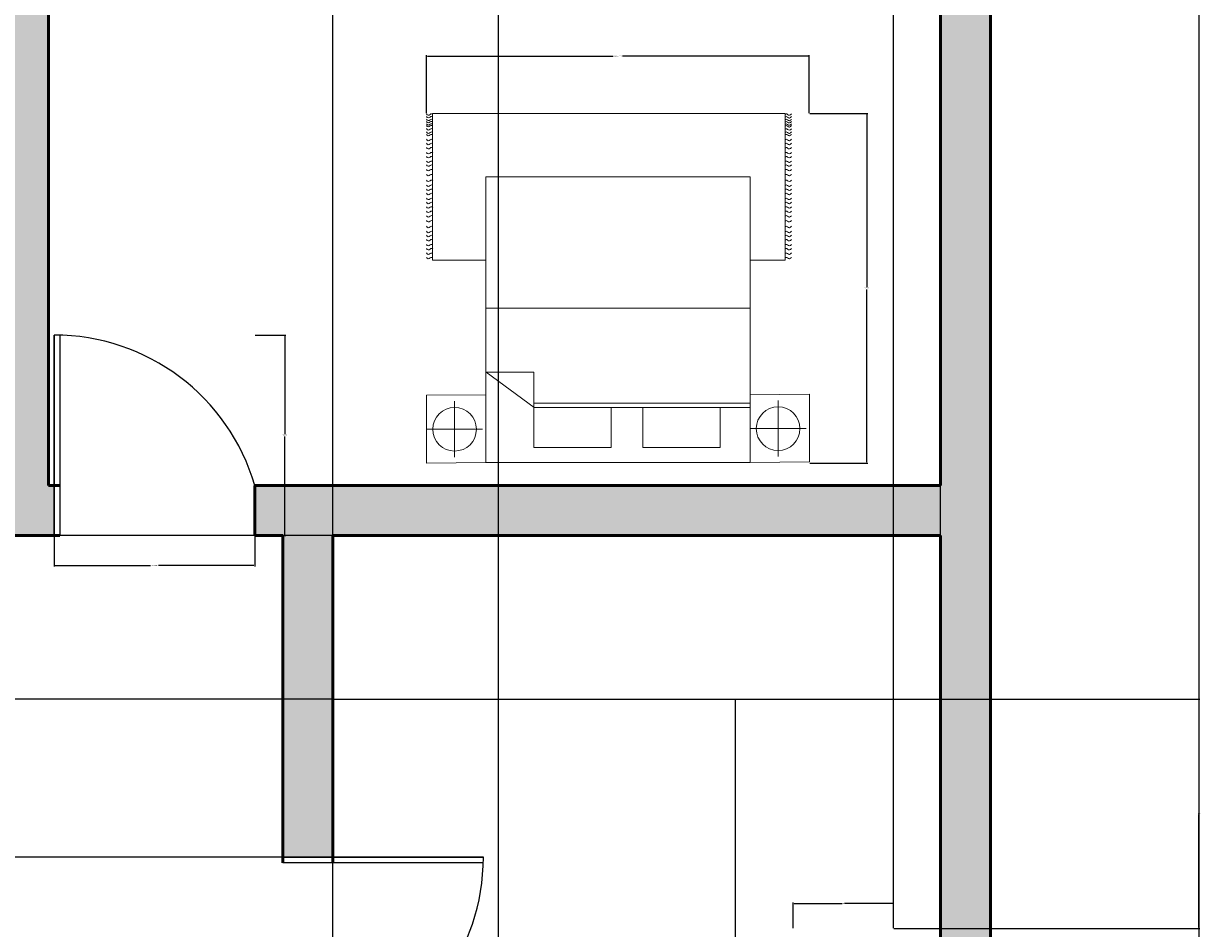
# Model space of a CAD drawing. Units: inches. Extents: x 383 to 970, y 275 to 1088.
# Tile 10 of 11: x 759 to 970, y 713 to 875. Entities that reach past the tile are written whole.
import ezdxf

# ---------------------------------------------------------------- set-up
doc = ezdxf.new("R2010")
doc.units = ezdxf.units.IN
doc.header["$MEASUREMENT"] = 0
for name, color, linetype, lineweight in [('A-ANNO-DIMS', 2, 'Continuous', 18), ('A-DOOR', 3, 'Continuous', 25), ('A-FLOR-CASE', 8, 'Continuous', 25), ('A-FURN', 8, 'Continuous', 18), ('A-WALL', 7, 'Continuous', 50)]:
    doc.layers.add(name, color=color, linetype=linetype, lineweight=lineweight)
doc.layers.add('A-WALL-PATT', color=251, linetype='Continuous', lineweight=13, true_color=0x636466)
doc.styles.get("Standard").update_dxf_attribs({"font": 'arial.ttf'})
doc.dimstyles.get("Standard").update_dxf_attribs({"dimtxt": 0.18, "dimasz": 0.18, "dimexe": 0.18, "dimexo": 0.0625, "dimgap": 0.09, "dimtad": 0, "dimtih": 1, "dimtoh": 1, "dimdec": 4, "dimzin": 0, "dimdsep": 46, "dimtxsty": 'Standard', "dimcen": 0.09, "dimadec": 0, "dimazin": 0, "dimtfac": 1, "dimtdec": 4, "dimtofl": 0, "dimtmove": 0, "dimatfit": 3, "dimfxl": 1, "dimtolj": 1, "dimtzin": 0, "dimarcsym": 0})

# ---------------------------------------------------------------- blocks, each defined once
blk = doc.blocks.new('BED-DOUBLE-WITH-NIGHTSTANDS')
for p, q in [((6.09, 68.68), (6.09, 58.62)), ((36.42, 67.59), (62.78, 67.59)), ((36.42, 58.05), (36.42, 67.59)), ((62.78, 67.59), (62.78, 4.35)), ((1.07, 63.65), (11.12, 63.65)), ((9.97, 49.39), (16.32, 58)), ((16.32, 49.44), (16.32, 58)), ((27.82, 58.05), (27.82, 10.63)), ((9.97, 49.44), (16.32, 49.44)), ((9.97, 49.39), (9.97, 10.63)), ((10.78, 49.44), (10.78, 10.63)), ((6.2, 10.63), (6.2, 0.57)), ((36.42, 4.35), (36.42, 10.65)), ((1.17, 5.6), (11.22, 5.6)), ((62.78, 4.35), (36.42, 4.35))]:
    blk.add_line(p, q)
for points in [[(12.29, 58.05), (12.19, 68.68), (0, 68.68), (0.1, 58.05)], [(0.1, 58.05), (51.42, 58.05), (51.42, 10.63), (0.1, 10.63)], [(2.8, 49.44), (9.97, 49.44), (9.97, 35.55), (2.8, 35.55)], [(2.8, 29.88), (9.97, 29.88), (9.97, 15.98), (2.8, 15.98)], [(12.39, 0), (12.29, 10.63), (0.1, 10.63), (0.21, 0)]]:
    blk.add_lwpolyline(points, close=True)
for centre in [(6.09, 63.65), (6.2, 5.6)]:
    blk.add_circle(centre, 3.92)
for points, knots in [([(36.95, 68.71), (36.83, 68.61), (36.59, 68.42), (36.83, 68.08), (37, 67.8), (36.89, 67.65), (36.85, 67.58)], [0, 0, 0, 0, 0.400747, 0.791423, 1.067667, 1.29709, 1.29709, 1.29709, 1.29709]), ([(37.73, 68.71), (37.61, 68.61), (37.37, 68.42), (37.61, 68.08), (37.78, 67.8), (37.67, 67.65), (37.62, 67.58)], [0, 0, 0, 0, 0.400747, 0.791423, 1.067667, 1.29709, 1.29709, 1.29709, 1.29709]), ([(38.54, 68.71), (38.42, 68.61), (38.18, 68.42), (38.42, 68.08), (38.59, 67.8), (38.49, 67.65), (38.44, 67.58)], [0, 0, 0, 0, 0.400747, 0.791423, 1.067667, 1.29709, 1.29709, 1.29709, 1.29709]), ([(39.27, 68.71), (39.15, 68.61), (38.91, 68.42), (39.15, 68.08), (39.32, 67.8), (39.22, 67.65), (39.17, 67.58)], [0, 0, 0, 0, 0.400747, 0.791423, 1.067667, 1.29709, 1.29709, 1.29709, 1.29709]), ([(40.15, 68.71), (40.03, 68.61), (39.79, 68.42), (40.03, 68.08), (40.21, 67.8), (40.1, 67.65), (40.05, 67.58)], [0, 0, 0, 0, 0.400747, 0.791423, 1.067667, 1.29709, 1.29709, 1.29709, 1.29709]), ([(40.91, 68.71), (40.78, 68.61), (40.54, 68.42), (40.78, 68.08), (40.96, 67.8), (40.85, 67.65), (40.8, 67.58)], [0, 0, 0, 0, 0.400747, 0.791423, 1.067667, 1.29709, 1.29709, 1.29709, 1.29709]), ([(41.63, 68.71), (41.51, 68.61), (41.27, 68.42), (41.51, 68.08), (41.69, 67.8), (41.58, 67.65), (41.53, 67.58)], [0, 0, 0, 0, 0.400747, 0.791423, 1.067667, 1.29709, 1.29709, 1.29709, 1.29709]), ([(42.52, 68.71), (42.39, 68.61), (42.16, 68.42), (42.39, 68.08), (42.57, 67.8), (42.46, 67.65), (42.41, 67.58)], [0, 0, 0, 0, 0.400747, 0.791423, 1.067667, 1.29709, 1.29709, 1.29709, 1.29709]), ([(43.55, 68.71), (43.43, 68.61), (43.19, 68.42), (43.43, 68.08), (43.6, 67.8), (43.5, 67.65), (43.45, 67.58)], [0, 0, 0, 0, 0.400747, 0.791423, 1.067667, 1.29709, 1.29709, 1.29709, 1.29709]), ([(44.43, 68.71), (44.31, 68.61), (44.07, 68.42), (44.31, 68.08), (44.49, 67.8), (44.38, 67.65), (44.33, 67.58)], [0, 0, 0, 0, 0.400747, 0.791423, 1.067667, 1.29709, 1.29709, 1.29709, 1.29709]), ([(45.25, 68.71), (45.13, 68.61), (44.89, 68.42), (45.13, 68.08), (45.3, 67.8), (45.2, 67.65), (45.15, 67.58)], [0, 0, 0, 0, 0.400747, 0.791423, 1.067667, 1.29709, 1.29709, 1.29709, 1.29709]), ([(46.03, 68.71), (45.91, 68.61), (45.67, 68.42), (45.91, 68.08), (46.08, 67.8), (45.97, 67.65), (45.92, 67.58)], [0, 0, 0, 0, 0.400747, 0.791423, 1.067667, 1.29709, 1.29709, 1.29709, 1.29709]), ([(46.84, 68.71), (46.72, 68.61), (46.48, 68.42), (46.72, 68.08), (46.9, 67.8), (46.79, 67.65), (46.74, 67.58)], [0, 0, 0, 0, 0.400747, 0.791423, 1.067667, 1.29709, 1.29709, 1.29709, 1.29709]), ([(47.57, 68.71), (47.45, 68.61), (47.21, 68.42), (47.45, 68.08), (47.62, 67.8), (47.52, 67.65), (47.47, 67.58)], [0, 0, 0, 0, 0.400747, 0.791423, 1.067667, 1.29709, 1.29709, 1.29709, 1.29709]), ([(48.45, 68.71), (48.33, 68.61), (48.09, 68.42), (48.33, 68.08), (48.51, 67.8), (48.4, 67.65), (48.35, 67.58)], [0, 0, 0, 0, 0.400747, 0.791423, 1.067667, 1.29709, 1.29709, 1.29709, 1.29709]), ([(49.21, 68.71), (49.08, 68.61), (48.85, 68.42), (49.08, 68.08), (49.26, 67.8), (49.15, 67.65), (49.1, 67.58)], [0, 0, 0, 0, 0.400747, 0.791423, 1.067667, 1.29709, 1.29709, 1.29709, 1.29709]), ([(49.93, 68.71), (49.81, 68.61), (49.57, 68.42), (49.81, 68.08), (49.99, 67.8), (49.88, 67.65), (49.83, 67.58)], [0, 0, 0, 0, 0.400747, 0.791423, 1.067667, 1.29709, 1.29709, 1.29709, 1.29709]), ([(50.82, 68.71), (50.69, 68.61), (50.46, 68.42), (50.69, 68.08), (50.87, 67.8), (50.76, 67.65), (50.71, 67.58)], [0, 0, 0, 0, 0.400747, 0.791423, 1.067667, 1.29709, 1.29709, 1.29709, 1.29709]), ([(51.85, 68.71), (51.73, 68.61), (51.49, 68.42), (51.73, 68.08), (51.9, 67.8), (51.8, 67.65), (51.75, 67.58)], [0, 0, 0, 0, 0.400747, 0.791423, 1.067667, 1.29709, 1.29709, 1.29709, 1.29709]), ([(52.74, 68.71), (52.61, 68.61), (52.37, 68.42), (52.61, 68.08), (52.79, 67.8), (52.68, 67.65), (52.63, 67.58)], [0, 0, 0, 0, 0.400747, 0.791423, 1.067667, 1.29709, 1.29709, 1.29709, 1.29709]), ([(53.55, 68.71), (53.43, 68.61), (53.19, 68.42), (53.43, 68.08), (53.6, 67.8), (53.5, 67.65), (53.45, 67.58)], [0, 0, 0, 0, 0.400747, 0.791423, 1.067667, 1.29709, 1.29709, 1.29709, 1.29709]), ([(54.24, 68.71), (54.12, 68.61), (53.88, 68.42), (54.12, 68.08), (54.29, 67.8), (54.19, 67.65), (54.14, 67.58)], [0, 0, 0, 0, 0.400747, 0.791423, 1.067667, 1.29709, 1.29709, 1.29709, 1.29709]), ([(55.06, 68.71), (54.94, 68.61), (54.7, 68.42), (54.94, 68.08), (55.11, 67.8), (55, 67.65), (54.95, 67.58)], [0, 0, 0, 0, 0.400747, 0.791423, 1.067667, 1.29709, 1.29709, 1.29709, 1.29709]), ([(55.78, 68.71), (55.66, 68.61), (55.42, 68.42), (55.66, 68.08), (55.84, 67.8), (55.73, 67.65), (55.68, 67.58)], [0, 0, 0, 0, 0.400747, 0.791423, 1.067667, 1.29709, 1.29709, 1.29709, 1.29709]), ([(56.67, 68.71), (56.55, 68.61), (56.31, 68.42), (56.55, 68.08), (56.72, 67.8), (56.61, 67.65), (56.56, 67.58)], [0, 0, 0, 0, 0.400747, 0.791423, 1.067667, 1.29709, 1.29709, 1.29709, 1.29709]), ([(57.42, 68.71), (57.3, 68.61), (57.06, 68.42), (57.3, 68.08), (57.47, 67.8), (57.36, 67.65), (57.32, 67.58)], [0, 0, 0, 0, 0.400747, 0.791423, 1.067667, 1.29709, 1.29709, 1.29709, 1.29709]), ([(58.15, 68.71), (58.03, 68.61), (57.79, 68.42), (58.03, 68.08), (58.2, 67.8), (58.1, 67.66), (58.05, 67.59)], [0, 0, 0, 0, 0.400747, 0.791423, 1.067667, 1.283686, 1.283686, 1.283686, 1.283686]), ([(59.03, 68.71), (58.91, 68.61), (58.67, 68.42), (58.91, 68.08), (59.08, 67.8), (58.98, 67.66), (58.93, 67.59)], [0, 0, 0, 0, 0.400747, 0.791423, 1.067667, 1.283686, 1.283686, 1.283686, 1.283686]), ([(59.46, 68.71), (59.34, 68.61), (59.09, 68.42), (59.34, 68.08), (59.51, 67.8), (59.41, 67.66), (59.36, 67.59)], [0, 0, 0, 0, 0.402903, 0.794912, 1.071156, 1.287177, 1.287177, 1.287177, 1.287177]), ([(60.05, 68.71), (59.93, 68.61), (59.69, 68.42), (59.93, 68.08), (60.1, 67.8), (60, 67.66), (59.96, 67.59)], [0, 0, 0, 0, 0.400747, 0.791423, 1.067667, 1.283686, 1.283686, 1.283686, 1.283686]), ([(60.63, 68.71), (60.51, 68.61), (60.27, 68.42), (60.51, 68.08), (60.68, 67.8), (60.58, 67.66), (60.53, 67.59)], [0, 0, 0, 0, 0.400747, 0.791423, 1.067667, 1.283686, 1.283686, 1.283686, 1.283686]), ([(60.94, 68.71), (60.82, 68.61), (60.58, 68.42), (60.81, 68.08), (60.99, 67.8), (60.89, 67.66), (60.84, 67.59)], [0, 0, 0, 0, 0.400747, 0.791423, 1.067667, 1.283686, 1.283686, 1.283686, 1.283686]), ([(61.36, 68.71), (61.23, 68.61), (60.99, 68.42), (61.23, 68.08), (61.41, 67.8), (61.3, 67.65), (61.25, 67.58)], [0, 0, 0, 0, 0.400747, 0.791423, 1.067667, 1.29709, 1.29709, 1.29709, 1.29709]), ([(61.75, 68.71), (61.63, 68.61), (61.39, 68.42), (61.63, 68.08), (61.8, 67.8), (61.7, 67.65), (61.65, 67.58)], [0, 0, 0, 0, 0.400747, 0.791423, 1.067667, 1.29709, 1.29709, 1.29709, 1.29709]), ([(62.24, 68.71), (62.12, 68.61), (61.88, 68.42), (62.12, 68.08), (62.29, 67.8), (62.18, 67.65), (62.13, 67.58)], [0, 0, 0, 0, 0.400747, 0.791423, 1.067667, 1.29709, 1.29709, 1.29709, 1.29709]), ([(62.71, 68.71), (62.59, 68.61), (62.35, 68.42), (62.59, 68.08), (62.76, 67.8), (62.66, 67.65), (62.61, 67.58)], [0, 0, 0, 0, 0.400747, 0.791423, 1.067667, 1.29709, 1.29709, 1.29709, 1.29709]), ([(36.95, 3.23), (36.83, 3.32), (36.59, 3.52), (36.83, 3.86), (37, 4.14), (36.89, 4.29), (36.85, 4.35)], [0, 0, 0, 0, 0.400747, 0.791423, 1.067667, 1.29709, 1.29709, 1.29709, 1.29709]), ([(37.73, 3.23), (37.61, 3.32), (37.37, 3.52), (37.61, 3.86), (37.78, 4.14), (37.67, 4.29), (37.62, 4.35)], [0, 0, 0, 0, 0.400747, 0.791423, 1.067667, 1.29709, 1.29709, 1.29709, 1.29709]), ([(38.54, 3.23), (38.42, 3.32), (38.18, 3.52), (38.42, 3.86), (38.59, 4.14), (38.49, 4.29), (38.44, 4.35)], [0, 0, 0, 0, 0.400747, 0.791423, 1.067667, 1.29709, 1.29709, 1.29709, 1.29709]), ([(39.27, 3.23), (39.15, 3.32), (38.91, 3.52), (39.15, 3.86), (39.32, 4.14), (39.22, 4.29), (39.17, 4.35)], [0, 0, 0, 0, 0.400747, 0.791423, 1.067667, 1.29709, 1.29709, 1.29709, 1.29709]), ([(40.15, 3.23), (40.03, 3.32), (39.79, 3.52), (40.03, 3.86), (40.21, 4.14), (40.1, 4.29), (40.05, 4.35)], [0, 0, 0, 0, 0.400747, 0.791423, 1.067667, 1.29709, 1.29709, 1.29709, 1.29709]), ([(40.91, 3.23), (40.78, 3.32), (40.54, 3.52), (40.78, 3.86), (40.96, 4.14), (40.85, 4.29), (40.8, 4.35)], [0, 0, 0, 0, 0.400747, 0.791423, 1.067667, 1.29709, 1.29709, 1.29709, 1.29709]), ([(41.63, 3.23), (41.51, 3.32), (41.27, 3.52), (41.51, 3.86), (41.69, 4.14), (41.58, 4.29), (41.53, 4.35)], [0, 0, 0, 0, 0.400747, 0.791423, 1.067667, 1.29709, 1.29709, 1.29709, 1.29709]), ([(42.52, 3.23), (42.39, 3.32), (42.16, 3.52), (42.39, 3.86), (42.57, 4.14), (42.46, 4.29), (42.41, 4.35)], [0, 0, 0, 0, 0.400747, 0.791423, 1.067667, 1.29709, 1.29709, 1.29709, 1.29709]), ([(43.55, 3.23), (43.43, 3.32), (43.19, 3.52), (43.43, 3.86), (43.6, 4.14), (43.5, 4.29), (43.45, 4.35)], [0, 0, 0, 0, 0.400747, 0.791423, 1.067667, 1.29709, 1.29709, 1.29709, 1.29709]), ([(44.43, 3.23), (44.31, 3.32), (44.07, 3.52), (44.31, 3.86), (44.49, 4.14), (44.38, 4.29), (44.33, 4.35)], [0, 0, 0, 0, 0.400747, 0.791423, 1.067667, 1.29709, 1.29709, 1.29709, 1.29709]), ([(45.25, 3.23), (45.13, 3.32), (44.89, 3.52), (45.13, 3.86), (45.3, 4.14), (45.2, 4.29), (45.15, 4.35)], [0, 0, 0, 0, 0.400747, 0.791423, 1.067667, 1.29709, 1.29709, 1.29709, 1.29709]), ([(46.03, 3.23), (45.91, 3.32), (45.67, 3.52), (45.91, 3.86), (46.08, 4.14), (45.97, 4.29), (45.92, 4.35)], [0, 0, 0, 0, 0.400747, 0.791423, 1.067667, 1.29709, 1.29709, 1.29709, 1.29709]), ([(46.84, 3.23), (46.72, 3.32), (46.48, 3.52), (46.72, 3.86), (46.9, 4.14), (46.79, 4.29), (46.74, 4.35)], [0, 0, 0, 0, 0.400747, 0.791423, 1.067667, 1.29709, 1.29709, 1.29709, 1.29709]), ([(47.57, 3.23), (47.45, 3.32), (47.21, 3.52), (47.45, 3.86), (47.62, 4.14), (47.52, 4.29), (47.47, 4.35)], [0, 0, 0, 0, 0.400747, 0.791423, 1.067667, 1.29709, 1.29709, 1.29709, 1.29709]), ([(48.45, 3.23), (48.33, 3.32), (48.09, 3.52), (48.33, 3.86), (48.51, 4.14), (48.4, 4.29), (48.35, 4.35)], [0, 0, 0, 0, 0.400747, 0.791423, 1.067667, 1.29709, 1.29709, 1.29709, 1.29709]), ([(49.21, 3.23), (49.08, 3.32), (48.85, 3.52), (49.08, 3.86), (49.26, 4.14), (49.15, 4.29), (49.1, 4.35)], [0, 0, 0, 0, 0.400747, 0.791423, 1.067667, 1.29709, 1.29709, 1.29709, 1.29709]), ([(49.93, 3.23), (49.81, 3.32), (49.57, 3.52), (49.81, 3.86), (49.99, 4.14), (49.88, 4.29), (49.83, 4.35)], [0, 0, 0, 0, 0.400747, 0.791423, 1.067667, 1.29709, 1.29709, 1.29709, 1.29709]), ([(50.82, 3.23), (50.69, 3.32), (50.46, 3.52), (50.69, 3.86), (50.87, 4.14), (50.76, 4.29), (50.71, 4.35)], [0, 0, 0, 0, 0.400747, 0.791423, 1.067667, 1.29709, 1.29709, 1.29709, 1.29709]), ([(51.85, 3.23), (51.73, 3.32), (51.49, 3.52), (51.73, 3.86), (51.9, 4.14), (51.8, 4.29), (51.75, 4.35)], [0, 0, 0, 0, 0.400747, 0.791423, 1.067667, 1.29709, 1.29709, 1.29709, 1.29709]), ([(52.74, 3.23), (52.61, 3.32), (52.37, 3.52), (52.61, 3.86), (52.79, 4.14), (52.68, 4.29), (52.63, 4.35)], [0, 0, 0, 0, 0.400747, 0.791423, 1.067667, 1.29709, 1.29709, 1.29709, 1.29709]), ([(53.55, 3.23), (53.43, 3.32), (53.19, 3.52), (53.43, 3.86), (53.6, 4.14), (53.5, 4.29), (53.45, 4.35)], [0, 0, 0, 0, 0.400747, 0.791423, 1.067667, 1.29709, 1.29709, 1.29709, 1.29709]), ([(54.24, 3.23), (54.12, 3.32), (53.88, 3.52), (54.12, 3.86), (54.29, 4.14), (54.19, 4.29), (54.14, 4.35)], [0, 0, 0, 0, 0.400747, 0.791423, 1.067667, 1.29709, 1.29709, 1.29709, 1.29709]), ([(55.06, 3.23), (54.94, 3.32), (54.7, 3.52), (54.94, 3.86), (55.11, 4.14), (55, 4.29), (54.95, 4.35)], [0, 0, 0, 0, 0.400747, 0.791423, 1.067667, 1.29709, 1.29709, 1.29709, 1.29709]), ([(55.78, 3.23), (55.66, 3.32), (55.42, 3.52), (55.66, 3.86), (55.84, 4.14), (55.73, 4.29), (55.68, 4.35)], [0, 0, 0, 0, 0.400747, 0.791423, 1.067667, 1.29709, 1.29709, 1.29709, 1.29709]), ([(56.67, 3.23), (56.55, 3.32), (56.31, 3.52), (56.55, 3.86), (56.72, 4.14), (56.61, 4.29), (56.56, 4.35)], [0, 0, 0, 0, 0.400747, 0.791423, 1.067667, 1.29709, 1.29709, 1.29709, 1.29709]), ([(57.42, 3.23), (57.3, 3.32), (57.06, 3.52), (57.3, 3.86), (57.47, 4.14), (57.36, 4.29), (57.32, 4.35)], [0, 0, 0, 0, 0.400747, 0.791423, 1.067667, 1.29709, 1.29709, 1.29709, 1.29709]), ([(58.15, 3.23), (58.03, 3.32), (57.79, 3.52), (58.03, 3.86), (58.2, 4.14), (58.09, 4.29), (58.04, 4.35)], [0, 0, 0, 0, 0.400747, 0.791423, 1.067667, 1.29709, 1.29709, 1.29709, 1.29709]), ([(59.03, 3.23), (58.91, 3.32), (58.67, 3.52), (58.91, 3.86), (59.08, 4.14), (58.98, 4.29), (58.93, 4.35)], [0, 0, 0, 0, 0.400747, 0.791423, 1.067667, 1.29709, 1.29709, 1.29709, 1.29709]), ([(59.46, 3.23), (59.33, 3.32), (59.08, 3.52), (59.34, 3.86), (59.51, 4.14), (59.4, 4.29), (59.36, 4.35)], [0, 0, 0, 0, 0.407265, 0.802015, 1.07826, 1.307683, 1.307683, 1.307683, 1.307683]), ([(60.03, 3.23), (59.9, 3.32), (59.67, 3.52), (59.9, 3.86), (60.08, 4.14), (59.97, 4.29), (59.92, 4.35)], [0, 0, 0, 0, 0.400747, 0.791423, 1.067667, 1.29709, 1.29709, 1.29709, 1.29709]), ([(60.6, 3.23), (60.48, 3.32), (60.24, 3.52), (60.48, 3.86), (60.65, 4.14), (60.54, 4.29), (60.5, 4.35)], [0, 0, 0, 0, 0.400747, 0.791423, 1.067667, 1.29709, 1.29709, 1.29709, 1.29709]), ([(60.91, 3.23), (60.79, 3.32), (60.55, 3.52), (60.79, 3.86), (60.96, 4.14), (60.85, 4.29), (60.81, 4.35)], [0, 0, 0, 0, 0.400747, 0.791423, 1.067667, 1.29709, 1.29709, 1.29709, 1.29709]), ([(61.33, 3.23), (61.21, 3.32), (60.97, 3.52), (61.21, 3.86), (61.38, 4.14), (61.27, 4.29), (61.22, 4.35)], [0, 0, 0, 0, 0.400747, 0.791423, 1.067667, 1.29709, 1.29709, 1.29709, 1.29709]), ([(61.72, 3.23), (61.6, 3.32), (61.36, 3.52), (61.6, 3.86), (61.78, 4.14), (61.67, 4.29), (61.62, 4.35)], [0, 0, 0, 0, 0.400747, 0.791423, 1.067667, 1.29709, 1.29709, 1.29709, 1.29709]), ([(62.21, 3.23), (62.09, 3.32), (61.85, 3.52), (62.09, 3.86), (62.26, 4.14), (62.16, 4.29), (62.11, 4.35)], [0, 0, 0, 0, 0.400747, 0.791423, 1.067667, 1.29709, 1.29709, 1.29709, 1.29709]), ([(62.71, 3.23), (62.59, 3.32), (62.35, 3.52), (62.59, 3.86), (62.76, 4.14), (62.66, 4.29), (62.61, 4.35)], [0, 0, 0, 0, 0.400747, 0.791423, 1.067667, 1.29709, 1.29709, 1.29709, 1.29709])]:
    blk.add_open_spline(points, degree=3, knots=knots)
blk = doc.blocks.new('DOOR-LEAF-36IN')
for p, q in [((0, 0), (0, 36)), ((1, 36), (1, 0)), ((0, 0), (1, 0))]:
    blk.add_line(p, q)
blk.add_arc((0, -1.5), 37.5, 16.2602, 90)
blk = doc.blocks.new('*D13')
at = {"layer": 'A-ANNO-DIMS', "color": 0, "lineweight": -2, "transparency": 16777216}
for p, q in [((764.24, 783.07), (764.24, 777.56)), ((800.24, 783.07), (800.24, 777.56)), ((764.42, 777.74), (781.52, 777.74)), ((800.06, 777.74), (782.96, 777.74))]:
    blk.add_line(p, q, dxfattribs=at)
at = {"layer": 'A-ANNO-DIMS', "color": 0, "transparency": 16777216}
for points in [[(764.42, 777.77), (764.42, 777.71), (764.24, 777.74)], [(800.06, 777.77), (800.06, 777.71), (800.24, 777.74)]]:
    blk.add_solid(points, dxfattribs=at)
at = {"layer": 'Defpoints', "color": 0, "transparency": 16777216}
for p in [(764.24, 783.14), (800.24, 783.14), (800.24, 777.74)]:
    blk.add_point(p, dxfattribs=at)
at = {"layer": 'A-ANNO-DIMS', "color": 0, "transparency": 16777216, "insert": (782.24, 777.74), "char_height": 0.18, "attachment_point": 5}
blk.add_mtext('\\A1;D1 36 TYP.', dxfattribs=at)
blk = doc.blocks.new('*D14')
at = {"layer": 'A-ANNO-DIMS', "color": 0, "lineweight": -2, "transparency": 16777216}
for p, q in [((800.3, 819.14), (805.82, 819.14)), ((805.64, 818.96), (805.64, 801.32)), ((805.64, 783.32), (805.64, 800.95)), ((800.3, 783.14), (805.82, 783.14))]:
    blk.add_line(p, q, dxfattribs=at)
at = {"layer": 'A-ANNO-DIMS', "color": 0, "transparency": 16777216}
for points in [[(805.61, 818.96), (805.67, 818.96), (805.64, 819.14)], [(805.61, 783.32), (805.67, 783.32), (805.64, 783.14)]]:
    blk.add_solid(points, dxfattribs=at)
at = {"layer": 'Defpoints', "color": 0, "transparency": 16777216}
for p in [(800.24, 819.14), (805.64, 819.14), (800.24, 783.14)]:
    blk.add_point(p, dxfattribs=at)
at = {"layer": 'A-ANNO-DIMS', "color": 0, "transparency": 16777216, "insert": (805.64, 801.14), "char_height": 0.18, "attachment_point": 5}
blk.add_mtext('\\A1;36 TYP.', dxfattribs=at)
blk = doc.blocks.new('*D25')
at = {"layer": 'A-ANNO-DIMS', "color": 0, "lineweight": -2, "transparency": 16777216}
for p, q in [((831.01, 858.98), (831.01, 869.4)), ((831.19, 869.22), (864.55, 869.22)), ((899.54, 869.22), (866.19, 869.22)), ((899.72, 858.98), (899.72, 869.4))]:
    blk.add_line(p, q, dxfattribs=at)
at = {"layer": 'A-ANNO-DIMS', "color": 0, "transparency": 16777216}
for points in [[(831.19, 869.25), (831.19, 869.19), (831.01, 869.22)], [(899.54, 869.25), (899.54, 869.19), (899.72, 869.22)]]:
    blk.add_solid(points, dxfattribs=at)
at = {"layer": 'Defpoints', "color": 0, "transparency": 16777216}
for p in [(831.01, 869.22), (831.01, 858.92), (899.72, 858.92)]:
    blk.add_point(p, dxfattribs=at)
at = {"layer": 'A-ANNO-DIMS', "color": 0, "transparency": 16777216, "insert": (865.37, 869.22), "char_height": 0.18, "attachment_point": 5}
blk.add_mtext('\\A1;BED 69 TYP.', dxfattribs=at)
blk = doc.blocks.new('*D26')
at = {"layer": 'A-ANNO-DIMS', "color": 0, "lineweight": -2, "transparency": 16777216}
for p, q in [((899.79, 858.92), (910.21, 858.92)), ((910.03, 858.74), (910.03, 827.71)), ((910.03, 796.31), (910.03, 827.34)), ((899.79, 796.13), (910.21, 796.13))]:
    blk.add_line(p, q, dxfattribs=at)
at = {"layer": 'A-ANNO-DIMS', "color": 0, "transparency": 16777216}
for points in [[(910, 858.74), (910.06, 858.74), (910.03, 858.92)], [(910, 796.31), (910.06, 796.31), (910.03, 796.13)]]:
    blk.add_solid(points, dxfattribs=at)
at = {"layer": 'Defpoints', "color": 0, "transparency": 16777216}
for p in [(899.72, 858.92), (910.03, 858.92), (899.72, 796.13)]:
    blk.add_point(p, dxfattribs=at)
at = {"layer": 'A-ANNO-DIMS', "color": 0, "transparency": 16777216, "insert": (910.03, 827.53), "char_height": 0.18, "attachment_point": 5}
blk.add_mtext('\\A1;63 TYP.', dxfattribs=at)
blk = doc.blocks.new('*D34')
at = {"layer": 'A-ANNO-DIMS', "color": 0, "lineweight": -2, "transparency": 16777216}
for p, q in [((896.83, 712.66), (896.83, 717.25)), ((897.01, 717.07), (905.6, 717.07)), ((914.62, 717.07), (906.02, 717.07)), ((914.8, 712.66), (914.8, 717.25))]:
    blk.add_line(p, q, dxfattribs=at)
at = {"layer": 'A-ANNO-DIMS', "color": 0, "transparency": 16777216}
for points in [[(897.01, 717.1), (897.01, 717.04), (896.83, 717.07)], [(914.62, 717.1), (914.62, 717.04), (914.8, 717.07)]]:
    blk.add_solid(points, dxfattribs=at)
at = {"layer": 'Defpoints', "color": 0, "transparency": 16777216}
for p in [(896.83, 717.07), (896.83, 712.6), (914.8, 712.6)]:
    blk.add_point(p, dxfattribs=at)
at = {"layer": 'A-ANNO-DIMS', "color": 0, "transparency": 16777216, "insert": (905.81, 717.07), "char_height": 0.18, "attachment_point": 5}
blk.add_mtext('\\A1;18', dxfattribs=at)
blk = doc.blocks.new('*D38')
at = {"layer": 'A-ANNO-DIMS', "color": 0, "lineweight": -2, "transparency": 16777216}
for p, q in [((932.3, 1050.14), (969.77, 1050.14)), ((969.59, 1049.96), (969.59, 681.32)), ((969.59, 312.32), (969.59, 680.95)), ((932.3, 312.14), (969.77, 312.14))]:
    blk.add_line(p, q, dxfattribs=at)
at = {"layer": 'A-ANNO-DIMS', "color": 0, "transparency": 16777216}
for points in [[(969.56, 1049.96), (969.62, 1049.96), (969.59, 1050.14)], [(969.56, 312.32), (969.62, 312.32), (969.59, 312.14)]]:
    blk.add_solid(points, dxfattribs=at)
at = {"layer": 'Defpoints', "color": 0, "transparency": 16777216}
for p in [(932.24, 1050.14), (969.59, 1050.14), (932.24, 312.14)]:
    blk.add_point(p, dxfattribs=at)
at = {"layer": 'A-ANNO-DIMS', "color": 0, "transparency": 16777216, "insert": (969.59, 681.14), "char_height": 0.18, "attachment_point": 5}
blk.add_mtext('\\A1;738', dxfattribs=at)
blk = doc.blocks.new('*D53')
at = {"layer": 'A-ANNO-DIMS', "color": 0, "lineweight": -2, "transparency": 16777216}
for p, q in [((814.18, 783.14), (382.71, 783.14)), ((382.89, 782.96), (382.89, 768.63)), ((382.89, 753.94), (382.89, 768.27)), ((814.18, 753.76), (382.71, 753.76))]:
    blk.add_line(p, q, dxfattribs=at)
at = {"layer": 'A-ANNO-DIMS', "color": 0, "transparency": 16777216}
for points in [[(382.86, 782.96), (382.92, 782.96), (382.89, 783.14)], [(382.86, 753.94), (382.92, 753.94), (382.89, 753.76)]]:
    blk.add_solid(points, dxfattribs=at)
at = {"layer": 'Defpoints', "color": 0, "transparency": 16777216}
for p in [(814.24, 783.14), (382.89, 753.76), (814.24, 753.76)]:
    blk.add_point(p, dxfattribs=at)
at = {"layer": 'A-ANNO-DIMS', "color": 0, "transparency": 16777216, "insert": (382.89, 768.45), "char_height": 0.18, "attachment_point": 5}
blk.add_mtext('\\A1;29.38', dxfattribs=at)
blk = doc.blocks.new('*D56')
at = {"layer": 'A-ANNO-DIMS', "color": 0, "lineweight": -2, "transparency": 16777216}
for p, q in [((805.18, 783.14), (382.71, 783.14)), ((382.89, 782.96), (382.89, 754.44)), ((382.89, 725.56), (382.89, 754.08)), ((805.18, 725.38), (382.71, 725.38))]:
    blk.add_line(p, q, dxfattribs=at)
at = {"layer": 'A-ANNO-DIMS', "color": 0, "transparency": 16777216}
for points in [[(382.86, 782.96), (382.92, 782.96), (382.89, 783.14)], [(382.86, 725.56), (382.92, 725.56), (382.89, 725.38)]]:
    blk.add_solid(points, dxfattribs=at)
at = {"layer": 'Defpoints', "color": 0, "transparency": 16777216}
for p in [(382.89, 783.14), (805.24, 783.14), (805.24, 725.38)]:
    blk.add_point(p, dxfattribs=at)
at = {"layer": 'A-ANNO-DIMS', "color": 0, "transparency": 16777216, "insert": (382.89, 754.26), "char_height": 0.18, "attachment_point": 5}
blk.add_mtext('\\A1;57.76', dxfattribs=at)
blk = doc.blocks.new('*D59')
at = {"layer": 'A-ANNO-DIMS', "color": 0, "lineweight": -2, "transparency": 16777216}
for p, q in [((814.24, 645.02), (814.24, 1087.67)), ((814.42, 1087.49), (828.65, 1087.49)), ((843.8, 1087.49), (829.58, 1087.49)), ((843.98, 640.59), (843.98, 1087.67))]:
    blk.add_line(p, q, dxfattribs=at)
at = {"layer": 'A-ANNO-DIMS', "color": 0, "transparency": 16777216}
for points in [[(814.42, 1087.52), (814.42, 1087.46), (814.24, 1087.49)], [(843.8, 1087.52), (843.8, 1087.46), (843.98, 1087.49)]]:
    blk.add_solid(points, dxfattribs=at)
at = {"layer": 'Defpoints', "color": 0, "transparency": 16777216}
for p in [(814.24, 1087.49), (814.24, 644.96), (843.98, 640.52)]:
    blk.add_point(p, dxfattribs=at)
at = {"layer": 'A-ANNO-DIMS', "color": 0, "transparency": 16777216, "insert": (829.11, 1087.49), "char_height": 0.18, "attachment_point": 5}
blk.add_mtext('\\A1;29.744', dxfattribs=at)
blk = doc.blocks.new('*D60')
at = {"layer": 'A-ANNO-DIMS', "color": 0, "lineweight": -2, "transparency": 16777216}
for p, q in [((886.47, 753.76), (969.77, 753.76)), ((969.59, 753.58), (969.59, 733.36)), ((969.59, 712.78), (969.59, 733)), ((914.86, 712.6), (969.77, 712.6))]:
    blk.add_line(p, q, dxfattribs=at)
at = {"layer": 'A-ANNO-DIMS', "color": 0, "transparency": 16777216}
for points in [[(969.56, 753.58), (969.62, 753.58), (969.59, 753.76)], [(969.56, 712.78), (969.62, 712.78), (969.59, 712.6)]]:
    blk.add_solid(points, dxfattribs=at)
at = {"layer": 'Defpoints', "color": 0, "transparency": 16777216}
for p in [(886.41, 753.76), (914.8, 712.6), (969.59, 712.6)]:
    blk.add_point(p, dxfattribs=at)
at = {"layer": 'A-ANNO-DIMS', "color": 0, "transparency": 16777216, "insert": (969.59, 733.18), "char_height": 0.18, "attachment_point": 5}
blk.add_mtext('\\A1;41.16', dxfattribs=at)
blk = doc.blocks.new('*D61')
at = {"layer": 'A-ANNO-DIMS', "color": 0, "lineweight": -2, "transparency": 16777216}
for p, q in [((914.8, 712.66), (914.8, 1087.67)), ((914.98, 1087.49), (918.63, 1087.49)), ((923.06, 1087.49), (919.41, 1087.49)), ((923.24, 783.2), (923.24, 1087.67))]:
    blk.add_line(p, q, dxfattribs=at)
at = {"layer": 'A-ANNO-DIMS', "color": 0, "transparency": 16777216}
for points in [[(914.98, 1087.52), (914.98, 1087.46), (914.8, 1087.49)], [(923.06, 1087.52), (923.06, 1087.46), (923.24, 1087.49)]]:
    blk.add_solid(points, dxfattribs=at)
at = {"layer": 'Defpoints', "color": 0, "transparency": 16777216}
for p in [(923.24, 1087.49), (923.24, 783.14), (914.8, 712.6)]:
    blk.add_point(p, dxfattribs=at)
at = {"layer": 'A-ANNO-DIMS', "color": 0, "transparency": 16777216, "insert": (919.02, 1087.49), "char_height": 0.18, "attachment_point": 5}
blk.add_mtext('\\A1;8.439', dxfattribs=at)

msp = doc.modelspace()

# ---------------------------------------------------------------- hatches: boundary and pattern name
at = {"layer": 'A-WALL-PATT'}
h = msp.add_hatch(color=256, dxfattribs=at)
h.dxf.hatch_style = 1
h.paths.add_polyline_path([(651.24, 321.1365), (651.24, 417.1365), (735.24, 417.1365), (735.24, 491.9233), (726.24, 491.9233), (726.24, 426.1365), (582.24, 426.1365), (582.24, 606.1365), (687.24, 606.1365), (687.24, 615.1365), (573.24, 615.1365), (573.24, 546.1365), (570.24, 546.1365), (570.24, 537.1365), (573.24, 537.1365), (573.24, 414.1365), (582.24, 414.1365), (582.24, 417.1365), (642.24, 417.1365), (642.24, 321.1365), (621.6203, 321.1365), (621.6203, 312.1365), (651.24, 312.1365)], flags=17)
h.paths.add_polyline_path([(597.6203, 321.1365), (582.24, 321.1365), (582.24, 390.1365), (573.24, 390.1365), (573.24, 321.1365), (570.24, 321.1365), (570.24, 312.1365), (573.24, 312.1365), (597.6203, 312.1365)], flags=16)
h.paths.add_polyline_path([(534.24, 321.1365), (500.8868, 321.1365), (500.8868, 312.1365), (534.24, 312.1365)], flags=17)
h.paths.add_polyline_path([(735.24, 606.1365), (738.24, 606.1365), (738.24, 615.1365), (723.24, 615.1365), (723.24, 606.1365), (726.24, 606.1365), (726.24, 551.9233), (735.24, 551.9233)], flags=17)
h.paths.add_polyline_path([(848.0899, 615.1365), (814.24, 615.1365), (814.24, 689.38), (805.24, 689.38), (805.24, 615.1365), (802.24, 615.1365), (802.24, 606.1365), (848.0899, 606.1365)], flags=17)
h.paths.add_polyline_path([(530.24, 615.1365), (498.24, 615.1365), (498.24, 646.5351), (489.24, 646.5351), (489.24, 615.1365), (466.771, 615.1365), (466.771, 606.1365), (521.24, 606.1365), (521.24, 603.1365), (530.24, 603.1365), (530.24, 606.1365)], flags=17)
h.paths.add_polyline_path([(498.24, 744.1365), (489.24, 744.1365), (489.24, 706.5351), (498.24, 706.5351)], flags=17)
h.paths.add_polyline_path([(715.24, 792.1365), (598.24, 792.1365), (598.24, 972.1365), (636.5058, 972.1365), (636.5058, 981.1365), (589.24, 981.1365), (589.24, 972.1365), (589.24, 792.1365), (586.24, 792.1365), (586.24, 783.1365), (589.24, 783.1365), (715.24, 783.1365)], flags=17)
h.paths.add_polyline_path([(763.24, 981.1365), (696.5058, 981.1365), (696.5058, 972.1365), (754.24, 972.1365), (754.24, 792.1365), (751.24, 792.1365), (751.24, 783.1365), (754.24, 783.1365), (764.24, 783.1365), (764.24, 792.1365), (763.24, 792.1365)], flags=17)
h.paths.add_polyline_path([(815.24, 1001.9492), (806.24, 1001.9492), (806.24, 972.1365), (818.24, 972.1365), (818.24, 981.1365), (815.24, 981.1365)], flags=17)
h.paths.add_polyline_path([(546.24, 1004.0336), (537.24, 1004.0336), (537.24, 981.1365), (534.24, 981.1365), (534.24, 972.1365), (537.24, 972.1365), (546.24, 972.1365), (546.24, 981.1365)], flags=17)
h.paths.add_polyline_path([(884.0899, 606.1365), (932.24, 606.1365), (932.24, 1050.1365), (420.24, 1050.1365), (420.24, 312.1365), (440.8868, 312.1365), (440.8868, 321.1365), (429.24, 321.1365), (429.24, 537.1365), (538.24, 537.1365), (538.24, 546.1365), (530.24, 546.1365), (530.24, 579.1365), (521.24, 579.1365), (521.24, 546.1365), (429.24, 546.1365), (429.24, 606.1365), (442.771, 606.1365), (442.771, 615.1365), (429.24, 615.1365), (429.24, 783.1365), (489.24, 783.1365), (489.24, 780.1365), (498.24, 780.1365), (498.24, 783.1365), (550.24, 783.1365), (550.24, 792.1365), (429.24, 792.1365), (429.24, 972.1365), (510.24, 972.1365), (510.24, 981.1365), (429.24, 981.1365), (429.24, 1041.1365), (537.24, 1041.1365), (537.24, 1028.0336), (546.24, 1028.0336), (546.24, 1041.1365), (806.24, 1041.1365), (806.24, 1025.9492), (815.24, 1025.9492), (815.24, 1041.1365), (923.24, 1041.1365), (923.24, 981.1365), (842.24, 981.1365), (842.24, 972.1365), (923.24, 972.1365), (923.24, 792.1365), (800.24, 792.1365), (800.24, 783.1365), (805.24, 783.1365), (805.24, 725.38), (814.24, 725.38), (814.24, 783.1365), (923.24, 783.1365), (923.24, 615.1365), (884.0899, 615.1365)])

# ---------------------------------------------------------------- linework, layer by layer
at = {"layer": 'A-DOOR'}
for p, q in [((764.24, 819.1365), (764.24, 783.1365)), ((841.24, 725.38), (805.24, 725.38))]:
    msp.add_line(p, q, dxfattribs=at)
at = {"layer": 'A-FLOR-CASE'}
for p, q in [((814.24, 753.7583), (886.4057, 753.7583)), ((886.4057, 753.7583), (886.4057, 644.9565))]:
    msp.add_line(p, q, dxfattribs=at)
at = {"layer": 'A-WALL'}
for p, q in [((932.24, 1050.1365), (932.24, 312.1365)), ((763.24, 981.1365), (763.24, 792.1365)), ((923.24, 972.1365), (923.24, 792.1365)), ((763.24, 792.1365), (765.24, 792.1365)), ((800.24, 783.1365), (800.24, 792.1365)), ((800.24, 792.1365), (923.24, 792.1365)), ((750.24, 783.1365), (765.24, 783.1365)), ((763.24, 783.1365), (764.24, 783.1365)), ((800.24, 783.1365), (805.24, 783.1365)), ((805.24, 783.1365), (805.24, 724.38)), ((814.24, 783.1365), (814.24, 724.38)), ((814.24, 783.1365), (923.24, 783.1365)), ((923.24, 783.1365), (923.24, 615.1365))]:
    msp.add_line(p, q, dxfattribs=at)

# ---------------------------------------------------------------- block references
at = {"layer": 'A-DOOR'}
msp.add_blockref('DOOR-LEAF-36IN', (764.24, 783.136), dxfattribs=at)
at = {"layer": 'A-DOOR', "rotation": 270}
msp.add_blockref('DOOR-LEAF-36IN', (805.2396, 725.3801), dxfattribs=at)
at = {"layer": 'A-FURN', "rotation": 89.99999999999717}
msp.add_blockref('BED-DOUBLE-WITH-NIGHTSTANDS', (899.7236, 796.1341), dxfattribs=at)

# ---------------------------------------------------------------- dimensions: what is measured, and where the dimension line sits
at = {"layer": 'A-ANNO-DIMS'}
for base, p1, p2, picture, middle in [((814.24, 1087.4865), (843.9841, 640.5231), (814.24, 644.9565), '*D59', (829.1121, 1087.4865)), ((923.24, 1087.4865), (914.8009, 712.601), (923.24, 783.1365), '*D61', (919.0205, 1087.4865))]:
    dim = msp.add_linear_dim(base=base, p1=p1, p2=p2, dimstyle='Standard', override={"dimdec": 3, "dimlfac": 1, "dimrnd": 0, "dimzin": 0, "dimdsep": 46, "dimlunit": 2}, dxfattribs=at)
    dim.commit()
    dim.dimension.update_dxf_attribs({"geometry": picture, "text_midpoint": middle})
for base, p1, p2, angle, override, picture, middle in [((969.59, 1050.1365), (932.24, 312.1365), (932.24, 1050.1365), 90, {"dimdec": 0, "dimlfac": 1, "dimrnd": 0, "dimzin": 0, "dimdsep": 46, "dimlunit": 2}, '*D38', (969.59, 681.1365)), ((382.89, 753.7583), (814.24, 783.1365), (814.24, 753.7583), 90, {"dimdec": 2, "dimlfac": 1, "dimrnd": 0, "dimzin": 0, "dimdsep": 46, "dimlunit": 2}, '*D53', (382.89, 768.4474)), ((382.89, 783.1365), (805.24, 725.38), (805.24, 783.1365), 90, {"dimdec": 2, "dimlfac": 1, "dimrnd": 0, "dimzin": 0, "dimdsep": 46, "dimlunit": 2}, '*D56', (382.89, 754.2583)), ((969.59, 712.601), (886.4057, 753.7583), (914.8009, 712.601), 90, {"dimdec": 2, "dimlfac": 1, "dimrnd": 0, "dimzin": 0, "dimdsep": 46, "dimlunit": 2}, '*D60', (969.59, 733.1796)), ((896.8275, 717.0724), (914.8009, 712.601), (896.8275, 712.601), 180, {"dimdec": 0, "dimlfac": 1, "dimrnd": 0, "dimzin": 0, "dimdsep": 46, "dimlunit": 2}, '*D34', (905.8142, 717.0724))]:
    dim = msp.add_linear_dim(base=base, p1=p1, p2=p2, angle=angle, dimstyle='Standard', override=override, dxfattribs=at)
    dim.commit()
    dim.dimension.update_dxf_attribs({"geometry": picture, "text_midpoint": middle})
for base, p1, p2, angle, text, picture, middle in [((831.0135, 869.2245), (899.7235, 858.918), (831.0135, 858.918), 180, 'BED <> TYP.', '*D25', (865.3685, 869.2245)), ((910.0299, 858.918), (899.7235, 796.1345), (899.7235, 858.918), 90, '<> TYP.', '*D26', (910.0299, 827.5263)), ((805.64, 819.1365), (800.24, 783.1365), (800.24, 819.1365), 90, '<> TYP.', '*D14', (805.64, 801.1365))]:
    dim = msp.add_linear_dim(base=base, p1=p1, p2=p2, angle=angle, text=text, dimstyle='Standard', override={"dimdec": 0, "dimlfac": 1, "dimrnd": 0, "dimzin": 0, "dimdsep": 46, "dimlunit": 2}, dxfattribs=at)
    dim.commit()
    dim.dimension.update_dxf_attribs({"geometry": picture, "text_midpoint": middle})
dim = msp.add_linear_dim(base=(800.24, 777.7365), p1=(764.24, 783.1365), p2=(800.24, 783.1365), text='D1 <> TYP.', dimstyle='Standard', override={"dimdec": 0, "dimlfac": 1, "dimrnd": 0, "dimzin": 0, "dimdsep": 46, "dimlunit": 2}, dxfattribs=at)
dim.commit()
dim.dimension.update_dxf_attribs({"geometry": '*D13', "text_midpoint": (782.24, 777.7365)})

doc.saveas('drawing.dxf')
